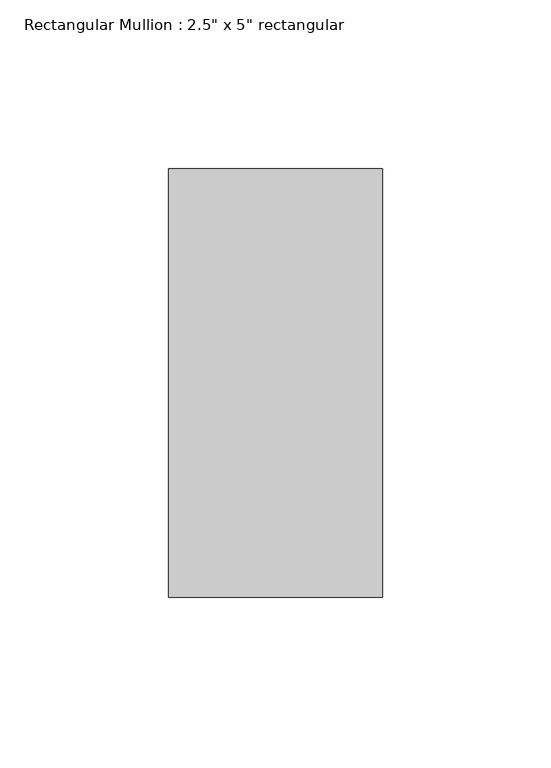
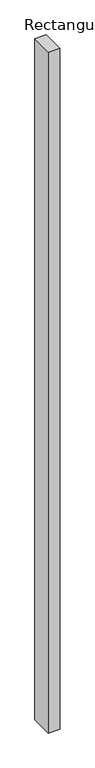
"""IFC4 building model written with IfcOpenShell, lengths in millimetres: member geometry."""

from ifc_helpers import new_model, si_unit, frame, origin, place, context, project, spatial, polyline, outline, extrude, source, transform, mapped, element, save


def member_fc36c840(model_context):
    return source(origin(), model_context, "Body", "SweptSolid", [
        extrude(outline(polyline([(0.0, 63.5), (0.0, -63.5), (-63.5, -63.5), (-63.5, 63.5), (0.0, 63.5)])), frame((0.0, 0.0, -3951.2205189), z_axis=(0.0, 0.0, 1.0), x_axis=(1.0, 0.0, 0.0)), (0.0, 0.0, 1.0), 3951.2205189),
    ])


if __name__ == "__main__":
    model = new_model("IFC4")
    model_context = context("Model", 3, world=origin())
    ifc_project = project(units=[si_unit("LENGTHUNIT", "METRE", prefix="MILLI")], contexts=[model_context])
    site = spatial("IfcSite", under=ifc_project)
    building = spatial("IfcBuilding", under=site)
    placement = place(None, origin())
    member_shape = member_fc36c840(model_context)
    element("IfcMember", 1, ObjectType="Rectangular Mullion : 2.5\" x 5\" rectangular", at=placement, inside=building, context=model_context, shape_type="MappedRepresentation", body=[
        mapped(member_shape, transform((0.0, 0.0, 0.0), x_axis=(1.0, 0.0, 0.0), y_axis=(0.0, 1.0, 0.0), z_axis=(0.0, 0.0, 1.0))),
    ])
    save(model, "model.ifc")

# Revit data of these elements
# Type "Rectangular Mullion : 2.5\" x 5\" rectangular"
#   built-in parameter 1007304 = 0.416667 (stored number, unit not read)
#   built-in parameter 1007301 = 0.104167 (stored number, unit not read)
#   built-in parameter 1007300 = 0.104167 (stored number, unit not read)
# Element 1 (IfcMember, "Rectangular Mullion : 2.5\" x 5\" rectangular")
#   Materials on its faces: "Aluminum"
# Materials
#   "Aluminum": class "Metal", colour RGB 247 247 247, transparency 0, Description = "Aluminum 6061", Cost = 0
